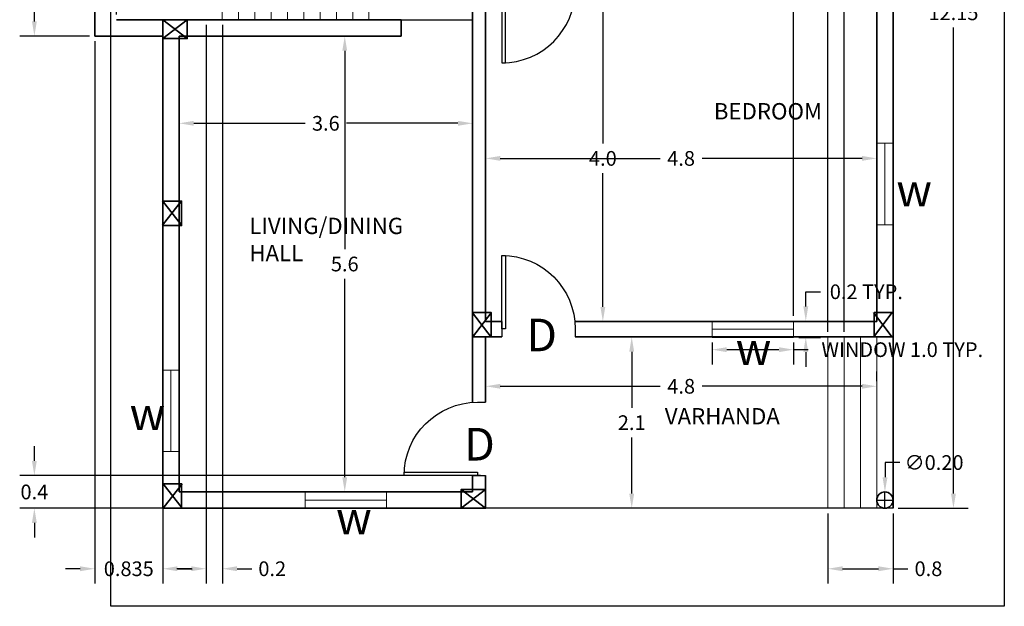
# Model space of a CAD drawing. Units: metres. Extents: x -16.7 to -4.6, y 24.4 to 40.
# Tile 1 of 2: x -16.7 to -4.6, y 24.4 to 31.6. Entities that reach past the tile are written whole.
import ezdxf

# ---------------------------------------------------------------- set-up
doc = ezdxf.new("R2010")
doc.units = ezdxf.units.M
doc.header["$MEASUREMENT"] = 0
doc.linetypes.add('ACAD_ISO02W100', pattern=[15, 12, -3])
for name, color, linetype, lineweight in [('A-ANNO-DIMS', 1, 'Continuous', 13), ('A-ANNO-TEXT', 5, 'Continuous', 18), ('A-ANNO-TTLB', 7, 'Continuous', 25), ('A-AREA-IDEN', 5, 'Continuous', 18), ('A-COLS', 7, 'Continuous', 35), ('A-FLOR', 4, 'Continuous', 25), ('A-WALL', 4, 'Continuous', 35), ('A-WALL-OVHD', 4, 'ACAD_ISO02W100', 25), ('door', 3, 'Continuous', 25), ('stair', 2, 'Continuous', 18), ('window', 6, 'Continuous', 20)]:
    doc.layers.add(name, color=color, linetype=linetype, lineweight=lineweight)
doc.styles.get("Standard").update_dxf_attribs({"font": 'arial.ttf'})
doc.dimstyles.get("Standard").update_dxf_attribs({"dimtxt": 0.18, "dimasz": 0.18, "dimexe": 0.18, "dimexo": 0.0625, "dimgap": 0.09, "dimtad": 0, "dimtih": 1, "dimtoh": 1, "dimdec": 1, "dimzin": 0, "dimdsep": 46, "dimtxsty": 'Standard', "dimcen": 0.09, "dimadec": 0, "dimazin": 0, "dimtfac": 1, "dimtdec": 1, "dimtofl": 0, "dimtmove": 0, "dimatfit": 3, "dimfxl": 1, "dimtolj": 1, "dimtzin": 0, "dimarcsym": 0})

# ---------------------------------------------------------------- blocks, each defined once
blk = doc.blocks.new('*U3')
for p, q in [((0, 0), (0, 100)), ((900, 0), (900, 100))]:
    blk.add_line(p, q)
blk.add_lwpolyline([(0, 0), (0, -900), (43.75, -900), (43.75, 0)], close=True)
blk.add_arc((0, 0), 900, 270, 0)
blk = doc.blocks.new('*U4')
for p, q in [((0, 0), (0, -100)), ((-900, 0), (-900, -100))]:
    blk.add_line(p, q)
blk.add_lwpolyline([(0, 0), (0, 900), (-43.75, 900), (-43.75, 0)], close=True)
blk.add_arc((0, 0), 900, 90, 180)
blk = doc.blocks.new('*D11')
at = {"layer": 'A-ANNO-DIMS', "color": 0, "lineweight": -2, "transparency": 16777216}
for p, q in [((-10.978, 29.979), (-10.978, 30.096)), ((-6.179, 29.979), (-6.179, 30.096)), ((-10.798, 29.916), (-8.836, 29.916)), ((-6.359, 29.916), (-8.321, 29.916))]:
    blk.add_line(p, q, dxfattribs=at)
at = {"layer": 'A-ANNO-DIMS', "color": 0, "transparency": 16777216}
for points in [[(-10.798, 29.946), (-10.798, 29.886), (-10.978, 29.916)], [(-6.359, 29.946), (-6.359, 29.886), (-6.179, 29.916)]]:
    blk.add_solid(points, dxfattribs=at)
at = {"layer": 'Defpoints', "color": 0, "transparency": 16777216}
for p in [(-10.978, 29.916), (-6.179, 29.916), (-6.179, 29.916)]:
    blk.add_point(p, dxfattribs=at)
at = {"layer": 'A-ANNO-DIMS', "color": 0, "transparency": 16777216, "insert": (-8.579, 29.916), "char_height": 0.18, "attachment_point": 5}
blk.add_mtext('\\A1;4.8', dxfattribs=at)
blk = doc.blocks.new('*D12')
at = {"layer": 'A-ANNO-DIMS', "color": 0, "lineweight": -2, "transparency": 16777216}
for p, q in [((-9.041, 31.916), (-9.719, 31.916)), ((-9.539, 31.736), (-9.539, 30.098)), ((-9.539, 28.096), (-9.539, 29.735)), ((-9.041, 27.916), (-9.719, 27.916))]:
    blk.add_line(p, q, dxfattribs=at)
at = {"layer": 'A-ANNO-DIMS', "color": 0, "transparency": 16777216}
for points in [[(-9.569, 31.736), (-9.509, 31.736), (-9.539, 31.916)], [(-9.569, 28.096), (-9.509, 28.096), (-9.539, 27.916)]]:
    blk.add_solid(points, dxfattribs=at)
at = {"layer": 'Defpoints', "color": 0, "transparency": 16777216}
for p in [(-8.978, 31.916), (-9.539, 27.916), (-8.978, 27.916)]:
    blk.add_point(p, dxfattribs=at)
at = {"layer": 'A-ANNO-DIMS', "color": 0, "transparency": 16777216, "insert": (-9.539, 29.916), "char_height": 0.18, "attachment_point": 5}
blk.add_mtext('\\A1;4.0', dxfattribs=at)
blk = doc.blocks.new('*D13')
at = {"layer": 'A-ANNO-DIMS', "color": 0, "lineweight": -2, "transparency": 16777216}
for p, q in [((-9.248, 27.726), (-9.365, 27.726)), ((-9.185, 27.546), (-9.185, 26.857)), ((-9.185, 25.806), (-9.185, 26.496)), ((-9.248, 25.626), (-9.365, 25.626))]:
    blk.add_line(p, q, dxfattribs=at)
at = {"layer": 'A-ANNO-DIMS', "color": 0, "transparency": 16777216}
for points in [[(-9.215, 27.546), (-9.155, 27.546), (-9.185, 27.726)], [(-9.215, 25.806), (-9.155, 25.806), (-9.185, 25.626)]]:
    blk.add_solid(points, dxfattribs=at)
at = {"layer": 'Defpoints', "color": 0, "transparency": 16777216}
for p in [(-9.185, 27.726), (-9.185, 25.626), (-9.185, 25.626)]:
    blk.add_point(p, dxfattribs=at)
at = {"layer": 'A-ANNO-DIMS', "color": 0, "transparency": 16777216, "insert": (-9.185, 26.676), "char_height": 0.18, "attachment_point": 5}
blk.add_mtext('\\A1;2.1', dxfattribs=at)
blk = doc.blocks.new('*D14')
at = {"layer": 'A-ANNO-DIMS', "color": 0, "lineweight": -2, "transparency": 16777216}
for p, q in [((-10.978, 27.185), (-10.978, 27.302)), ((-6.178, 27.185), (-6.178, 27.302)), ((-10.798, 27.122), (-8.836, 27.122)), ((-6.358, 27.122), (-8.321, 27.122))]:
    blk.add_line(p, q, dxfattribs=at)
at = {"layer": 'A-ANNO-DIMS', "color": 0, "transparency": 16777216}
for points in [[(-10.798, 27.152), (-10.798, 27.092), (-10.978, 27.122)], [(-6.358, 27.152), (-6.358, 27.092), (-6.178, 27.122)]]:
    blk.add_solid(points, dxfattribs=at)
at = {"layer": 'Defpoints', "color": 0, "transparency": 16777216}
for p in [(-10.978, 27.122), (-6.178, 27.122), (-6.178, 27.122)]:
    blk.add_point(p, dxfattribs=at)
at = {"layer": 'A-ANNO-DIMS', "color": 0, "transparency": 16777216, "insert": (-8.578, 27.122), "char_height": 0.18, "attachment_point": 5}
blk.add_mtext('\\A1;4.8', dxfattribs=at)
blk = doc.blocks.new('*D15')
at = {"layer": 'A-ANNO-DIMS', "color": 0, "lineweight": -2, "transparency": 16777216}
for p, q in [((-13.072, 31.416), (-12.526, 31.416)), ((-12.706, 31.236), (-12.706, 28.803)), ((-12.706, 26.006), (-12.706, 28.44)), ((-13.072, 25.826), (-12.526, 25.826))]:
    blk.add_line(p, q, dxfattribs=at)
at = {"layer": 'A-ANNO-DIMS', "color": 0, "transparency": 16777216}
for points in [[(-12.736, 31.236), (-12.676, 31.236), (-12.706, 31.416)], [(-12.736, 26.006), (-12.676, 26.006), (-12.706, 25.826)]]:
    blk.add_solid(points, dxfattribs=at)
at = {"layer": 'Defpoints', "color": 0, "transparency": 16777216}
for p in [(-13.135, 31.416), (-13.135, 25.826), (-12.706, 25.826)]:
    blk.add_point(p, dxfattribs=at)
at = {"layer": 'A-ANNO-DIMS', "color": 0, "transparency": 16777216, "insert": (-12.706, 28.621), "char_height": 0.18, "attachment_point": 5}
blk.add_mtext('\\A1;5.6', dxfattribs=at)
blk = doc.blocks.new('*D16')
at = {"layer": 'A-ANNO-DIMS', "color": 0, "lineweight": -2, "transparency": 16777216}
for p, q in [((-14.738, 30.098), (-14.738, 30.526)), ((-11.138, 30.098), (-11.138, 30.526)), ((-14.558, 30.346), (-13.192, 30.346)), ((-11.318, 30.346), (-12.685, 30.346))]:
    blk.add_line(p, q, dxfattribs=at)
at = {"layer": 'A-ANNO-DIMS', "color": 0, "transparency": 16777216}
for points in [[(-14.558, 30.376), (-14.558, 30.316), (-14.738, 30.346)], [(-11.318, 30.376), (-11.318, 30.316), (-11.138, 30.346)]]:
    blk.add_solid(points, dxfattribs=at)
at = {"layer": 'Defpoints', "color": 0, "transparency": 16777216}
for p in [(-11.138, 30.346), (-14.738, 30.036), (-11.138, 30.036)]:
    blk.add_point(p, dxfattribs=at)
at = {"layer": 'A-ANNO-DIMS', "color": 0, "transparency": 16777216, "insert": (-12.938, 30.346), "char_height": 0.18, "attachment_point": 5}
blk.add_mtext('\\A1;3.6', dxfattribs=at)
blk = doc.blocks.new('WIN-1000')
blk.add_line((0, 0.1), (1, 0.1))
blk.add_lwpolyline([(0, 0), (1, 0), (1, 0.2), (0, 0.2)], close=True)
blk = doc.blocks.new('COL-300x230')
for p, q in [((0, 0.23), (0.3, 0)), ((0, 0), (0.3, 0.23))]:
    blk.add_line(p, q)
blk.add_lwpolyline([(0, 0), (0, 0.23), (0.3, 0.23), (0.3, 0)], close=True)
blk = doc.blocks.new('STAIR-FLIGHT-2000x900')
for p, q in [((0.2, 0.9), (0.2, 0)), ((0.4, 0.9), (0.4, 0)), ((0.6, 0.9), (0.6, 0)), ((0.8, 0.9), (0.8, 0)), ((1, 0.9), (1, 0)), ((1.2, 0.9), (1.2, 0)), ((1.4, 0.9), (1.4, 0)), ((1.6, 0.9), (1.6, 0)), ((1.8, 0.9), (1.8, 0)), ((2, 0.9), (2, 0)), ((2, 0), (0, 0))]:
    blk.add_line(p, q)
blk = doc.blocks.new('*D23')
at = {"layer": 'A-ANNO-DIMS', "color": 0, "lineweight": -2, "transparency": 16777216}
for p, q in [((-8.199, 27.659), (-8.199, 27.391)), ((-8.019, 27.571), (-7.379, 27.571)), ((-7.199, 27.659), (-7.199, 27.391)), ((-7.199, 27.571), (-7.019, 27.571))]:
    blk.add_line(p, q, dxfattribs=at)
at = {"layer": 'A-ANNO-DIMS', "color": 0, "transparency": 16777216}
for points in [[(-8.019, 27.601), (-8.019, 27.541), (-8.199, 27.571)], [(-7.379, 27.601), (-7.379, 27.541), (-7.199, 27.571)]]:
    blk.add_solid(points, dxfattribs=at)
at = {"layer": 'Defpoints', "color": 0, "transparency": 16777216}
for p in [(-8.199, 27.721), (-7.199, 27.721), (-7.199, 27.571)]:
    blk.add_point(p, dxfattribs=at)
at = {"layer": 'A-ANNO-DIMS', "color": 0, "transparency": 16777216, "insert": (-5.865, 27.571), "char_height": 0.18, "attachment_point": 5}
blk.add_mtext('\\A1;WINDOW 1.0 TYP.', dxfattribs=at)
blk = doc.blocks.new('*D24')
at = {"layer": 'A-ANNO-DIMS', "color": 0, "lineweight": -2, "transparency": 16777216}
for p, q in [((-7.049, 28.101), (-7.049, 28.281)), ((-7.049, 28.281), (-6.869, 28.281)), ((-7.136, 27.921), (-6.869, 27.921)), ((-7.136, 27.721), (-6.869, 27.721)), ((-7.049, 27.541), (-7.049, 27.361))]:
    blk.add_line(p, q, dxfattribs=at)
at = {"layer": 'A-ANNO-DIMS', "color": 0, "transparency": 16777216}
for points in [[(-7.079, 28.101), (-7.019, 28.101), (-7.049, 27.921)], [(-7.079, 27.541), (-7.019, 27.541), (-7.049, 27.721)]]:
    blk.add_solid(points, dxfattribs=at)
at = {"layer": 'Defpoints', "color": 0, "transparency": 16777216}
for p in [(-7.199, 27.921), (-7.049, 27.921), (-7.199, 27.721)]:
    blk.add_point(p, dxfattribs=at)
at = {"layer": 'A-ANNO-DIMS', "color": 0, "transparency": 16777216, "insert": (-6.306, 28.281), "char_height": 0.18, "attachment_point": 5}
blk.add_mtext('\\A1;0.2 TYP.', dxfattribs=at)
blk = doc.blocks.new('*D32')
at = {"layer": 'A-ANNO-DIMS', "color": 0, "lineweight": -2, "transparency": 16777216}
for p, q in [((-5.916, 37.776), (-5.057, 37.776)), ((-5.237, 37.596), (-5.237, 31.883)), ((-5.237, 25.806), (-5.237, 31.52)), ((-5.916, 25.626), (-5.057, 25.626))]:
    blk.add_line(p, q, dxfattribs=at)
at = {"layer": 'A-ANNO-DIMS', "color": 0, "transparency": 16777216}
for points in [[(-5.267, 37.596), (-5.207, 37.596), (-5.237, 37.776)], [(-5.267, 25.806), (-5.207, 25.806), (-5.237, 25.626)]]:
    blk.add_solid(points, dxfattribs=at)
at = {"layer": 'Defpoints', "color": 0, "transparency": 16777216}
for p in [(-5.978, 37.776), (-5.237, 37.776), (-5.978, 25.626)]:
    blk.add_point(p, dxfattribs=at)
at = {"layer": 'A-ANNO-DIMS', "color": 0, "transparency": 16777216, "insert": (-5.237, 31.701), "char_height": 0.18, "attachment_point": 5}
blk.add_mtext('\\A1;12.15', dxfattribs=at)
blk = doc.blocks.new('*D33')
at = {"layer": 'A-ANNO-DIMS', "color": 0, "lineweight": -2, "transparency": 16777216}
for p, q in [((-15.773499, 31.353944), (-15.773499, 24.704754)), ((-14.938499, 31.353944), (-14.938499, 24.704754)), ((-15.953499, 24.884754), (-16.133499, 24.884754)), ((-14.758499, 24.884754), (-14.578499, 24.884754))]:
    blk.add_line(p, q, dxfattribs=at)
at = {"layer": 'A-ANNO-DIMS', "color": 0, "transparency": 16777216}
for points in [[(-15.953499, 24.914754), (-15.953499, 24.854754), (-15.773499, 24.884754)], [(-14.758499, 24.914754), (-14.758499, 24.854754), (-14.938499, 24.884754)]]:
    blk.add_solid(points, dxfattribs=at)
at = {"layer": 'Defpoints', "color": 0, "transparency": 16777216}
for p in [(-15.773499, 31.416444), (-14.938499, 31.416444), (-15.773499, 24.884754)]:
    blk.add_point(p, dxfattribs=at)
at = {"layer": 'A-ANNO-DIMS', "color": 0, "transparency": 16777216, "insert": (-15.355999, 24.884754), "char_height": 0.18, "attachment_point": 5}
blk.add_mtext('\\A1;0.835', dxfattribs=at)
blk = doc.blocks.new('*D34')
at = {"layer": 'A-ANNO-DIMS', "color": 0, "lineweight": -2, "transparency": 16777216}
for p, q in [((-15.836, 33.816), (-16.694, 33.816)), ((-16.514, 33.636), (-16.514, 32.797)), ((-16.514, 31.596), (-16.514, 32.436)), ((-15.836, 31.416), (-16.694, 31.416))]:
    blk.add_line(p, q, dxfattribs=at)
at = {"layer": 'A-ANNO-DIMS', "color": 0, "transparency": 16777216}
for points in [[(-16.544, 33.636), (-16.484, 33.636), (-16.514, 33.816)], [(-16.544, 31.596), (-16.484, 31.596), (-16.514, 31.416)]]:
    blk.add_solid(points, dxfattribs=at)
at = {"layer": 'Defpoints', "color": 0, "transparency": 16777216}
for p in [(-16.514, 33.816), (-15.773, 33.816), (-15.773, 31.416)]:
    blk.add_point(p, dxfattribs=at)
at = {"layer": 'A-ANNO-DIMS', "color": 0, "transparency": 16777216, "insert": (-16.514, 32.616), "char_height": 0.18, "attachment_point": 5}
blk.add_mtext('\\A1;2.4', dxfattribs=at)
blk = doc.blocks.new('*D35')
at = {"layer": 'A-ANNO-DIMS', "color": 0, "lineweight": -2, "transparency": 16777216}
for p, q in [((-15.508, 31.679), (-15.508, 38.697)), ((-14.408, 32.749), (-14.408, 38.697)), ((-15.328, 38.517), (-15.187, 38.517)), ((-14.588, 38.517), (-14.73, 38.517))]:
    blk.add_line(p, q, dxfattribs=at)
at = {"layer": 'A-ANNO-DIMS', "color": 0, "transparency": 16777216}
for points in [[(-15.328, 38.547), (-15.328, 38.487), (-15.508, 38.517)], [(-14.588, 38.547), (-14.588, 38.487), (-14.408, 38.517)]]:
    blk.add_solid(points, dxfattribs=at)
at = {"layer": 'Defpoints', "color": 0, "transparency": 16777216}
for p in [(-14.408, 38.517), (-14.408, 32.686), (-15.508, 31.616)]:
    blk.add_point(p, dxfattribs=at)
at = {"layer": 'A-ANNO-DIMS', "color": 0, "transparency": 16777216, "insert": (-14.958, 38.517), "char_height": 0.18, "attachment_point": 5}
blk.add_mtext('\\A1;1.1', dxfattribs=at)
blk = doc.blocks.new('*D36')
at = {"layer": 'A-ANNO-DIMS', "color": 0, "lineweight": -2, "transparency": 16777216}
for p, q in [((-14.408, 31.554), (-14.408, 24.705)), ((-14.208, 31.554), (-14.208, 24.705)), ((-14.588, 24.885), (-14.768, 24.885)), ((-14.028, 24.885), (-13.848, 24.885))]:
    blk.add_line(p, q, dxfattribs=at)
at = {"layer": 'A-ANNO-DIMS', "color": 0, "transparency": 16777216}
for points in [[(-14.588, 24.915), (-14.588, 24.855), (-14.408, 24.885)], [(-14.028, 24.915), (-14.028, 24.855), (-14.208, 24.885)]]:
    blk.add_solid(points, dxfattribs=at)
at = {"layer": 'Defpoints', "color": 0, "transparency": 16777216}
for p in [(-14.408, 31.616), (-14.208, 31.616), (-14.208, 24.885)]:
    blk.add_point(p, dxfattribs=at)
at = {"layer": 'A-ANNO-DIMS', "color": 0, "transparency": 16777216, "insert": (-13.596, 24.885), "char_height": 0.18, "attachment_point": 5}
blk.add_mtext('\\A1;0.2', dxfattribs=at)
blk = doc.blocks.new('*D37')
at = {"layer": 'A-ANNO-DIMS', "color": 0, "lineweight": -2, "transparency": 16777216}
for p, q in [((-6.778, 25.564), (-6.778, 24.705)), ((-5.978, 25.564), (-5.978, 24.705)), ((-6.598, 24.885), (-6.158, 24.885)), ((-5.978, 24.885), (-5.798, 24.885))]:
    blk.add_line(p, q, dxfattribs=at)
at = {"layer": 'A-ANNO-DIMS', "color": 0, "transparency": 16777216}
for points in [[(-6.598, 24.915), (-6.598, 24.855), (-6.778, 24.885)], [(-6.158, 24.915), (-6.158, 24.855), (-5.978, 24.885)]]:
    blk.add_solid(points, dxfattribs=at)
at = {"layer": 'Defpoints', "color": 0, "transparency": 16777216}
for p in [(-6.778, 25.626), (-5.978, 25.626), (-5.978, 24.885)]:
    blk.add_point(p, dxfattribs=at)
at = {"layer": 'A-ANNO-DIMS', "color": 0, "transparency": 16777216, "insert": (-5.544, 24.885), "char_height": 0.18, "attachment_point": 5}
blk.add_mtext('\\A1;0.8', dxfattribs=at)
blk = doc.blocks.new('*D38')
at = {"layer": 'A-ANNO-DIMS', "color": 0, "lineweight": -2, "transparency": 16777216}
for p, q in [((-6.778, 27.789), (-6.778, 38.697)), ((-6.578, 27.789), (-6.578, 38.697)), ((-6.958, 38.517), (-7.138, 38.517)), ((-6.398, 38.517), (-6.218, 38.517))]:
    blk.add_line(p, q, dxfattribs=at)
at = {"layer": 'A-ANNO-DIMS', "color": 0, "transparency": 16777216}
for points in [[(-6.958, 38.547), (-6.958, 38.487), (-6.778, 38.517)], [(-6.398, 38.547), (-6.398, 38.487), (-6.578, 38.517)]]:
    blk.add_solid(points, dxfattribs=at)
at = {"layer": 'Defpoints', "color": 0, "transparency": 16777216}
for p in [(-6.578, 38.517), (-6.778, 27.726), (-6.578, 27.726)]:
    blk.add_point(p, dxfattribs=at)
at = {"layer": 'A-ANNO-DIMS', "color": 0, "transparency": 16777216, "insert": (-5.966, 38.517), "char_height": 0.18, "attachment_point": 5}
blk.add_mtext('\\A1;0.2', dxfattribs=at)
blk = doc.blocks.new('*D39')
at = {"layer": 'A-ANNO-DIMS', "color": 0, "lineweight": -2, "transparency": 16777216}
for p, q in [((-7.199, 27.984), (-7.199, 38.697)), ((-6.178, 27.979), (-6.178, 38.697)), ((-7.379, 38.517), (-7.559, 38.517)), ((-5.998, 38.517), (-5.818, 38.517))]:
    blk.add_line(p, q, dxfattribs=at)
at = {"layer": 'A-ANNO-DIMS', "color": 0, "transparency": 16777216}
for points in [[(-7.379, 38.547), (-7.379, 38.487), (-7.199, 38.517)], [(-5.998, 38.547), (-5.998, 38.487), (-6.178, 38.517)]]:
    blk.add_solid(points, dxfattribs=at)
at = {"layer": 'Defpoints', "color": 0, "transparency": 16777216}
for p in [(-7.199, 38.517), (-7.199, 27.921), (-6.178, 27.916)]:
    blk.add_point(p, dxfattribs=at)
at = {"layer": 'A-ANNO-DIMS', "color": 0, "transparency": 16777216, "insert": (-6.689, 38.517), "char_height": 0.18, "attachment_point": 5}
blk.add_mtext('\\A1;1.02', dxfattribs=at)
blk = doc.blocks.new('*D40')
at = {"layer": 'A-ANNO-DIMS', "color": 0, "lineweight": -2, "transparency": 16777216}
for p, q in [((-16.514499, 26.206444), (-16.514499, 26.386444)), ((-11.040999, 26.026444), (-16.694499, 26.026444)), ((-11.040999, 25.626444), (-16.694499, 25.626444)), ((-16.514499, 25.446444), (-16.514499, 25.266444))]:
    blk.add_line(p, q, dxfattribs=at)
at = {"layer": 'A-ANNO-DIMS', "color": 0, "transparency": 16777216}
for points in [[(-16.544499, 26.206444), (-16.484499, 26.206444), (-16.514499, 26.026444)], [(-16.544499, 25.446444), (-16.484499, 25.446444), (-16.514499, 25.626444)]]:
    blk.add_solid(points, dxfattribs=at)
at = {"layer": 'Defpoints', "color": 0, "transparency": 16777216}
for p in [(-16.514499, 26.026444), (-10.978499, 26.026444), (-10.978499, 25.626444)]:
    blk.add_point(p, dxfattribs=at)
at = {"layer": 'A-ANNO-DIMS', "color": 0, "transparency": 16777216, "insert": (-16.514499, 25.826444), "char_height": 0.18, "attachment_point": 5}
blk.add_mtext('\\A1;0.4', dxfattribs=at)
blk = doc.blocks.new('*D44')
at = {"layer": 'A-ANNO-DIMS', "color": 0, "lineweight": -2, "transparency": 16777216}
for p, q in [((-6.076, 26.187), (-6.077, 26.007)), ((-5.896, 26.187), (-6.076, 26.187)), ((-6.078, 25.637), (-6.078, 25.817)), ((-6.168, 25.727), (-5.988, 25.727))]:
    blk.add_line(p, q, dxfattribs=at)
at = {"layer": 'A-ANNO-DIMS', "color": 0, "transparency": 16777216}
blk.add_solid([(-6.107, 26.007), (-6.047, 26.006), (-6.078, 25.827)], dxfattribs=at)
at = {"layer": 'Defpoints', "color": 0, "transparency": 16777216}
for p in [(-6.078, 25.827), (-6.079, 25.626)]:
    blk.add_point(p, dxfattribs=at)
at = {"layer": 'A-ANNO-DIMS', "color": 0, "transparency": 16777216, "insert": (-5.475, 26.187), "char_height": 0.18, "attachment_point": 5}
blk.add_mtext('\\A1;∅0.20', dxfattribs=at)

msp = doc.modelspace()

# ---------------------------------------------------------------- linework, layer by layer
at = {"layer": 'A-ANNO-TTLB'}
msp.add_lwpolyline([(-15.5749, 40.0289), (-4.6131, 40.0289), (-4.6131, 24.4246), (-15.5749, 24.4246)], close=True, dxfattribs=at)
at = {"layer": 'A-COLS'}
for p, q in [((-14.9393, 31.6146), (-14.6393, 31.3846)), ((-14.9393, 31.3846), (-14.6393, 31.6146)), ((-14.9403, 29.0962), (-14.7103, 29.3962)), ((-14.9403, 29.3962), (-14.7103, 29.0962)), ((-11.138, 27.7241), (-10.908, 28.0241)), ((-11.138, 28.0241), (-10.908, 27.7241)), ((-6.2183, 27.7262), (-5.9883, 28.0262)), ((-6.2183, 28.0262), (-5.9883, 27.7262)), ((-14.9328, 25.6258), (-14.7028, 25.9258)), ((-14.9328, 25.9258), (-14.7028, 25.6258))]:
    msp.add_line(p, q, dxfattribs=at)
for points in [[(-14.9386, 31.385), (-14.9386, 31.615), (-14.6386, 31.615), (-14.6386, 31.385)], [(-14.9385, 29.3932), (-14.7085, 29.3932), (-14.7085, 29.0932), (-14.9385, 29.0932)], [(-10.9085, 27.7264), (-11.1385, 27.7264), (-11.1385, 28.0264), (-10.9085, 28.0264)], [(-6.2085, 28.0264), (-5.9785, 28.0264), (-5.9785, 27.7264), (-6.2085, 27.7264)], [(-14.7085, 25.6264), (-14.9385, 25.6264), (-14.9385, 25.9264), (-14.7085, 25.9264)]]:
    msp.add_lwpolyline(points, close=True, dxfattribs=at)
msp.add_circle((-6.0785, 25.7265), 0.1001, dxfattribs=at)
at = {"layer": 'A-FLOR'}
msp.add_line((-5.9785, 25.6264), (-10.9785, 25.6264), dxfattribs=at)
at = {"layer": 'A-WALL'}
for p, q in [((-15.7735, 31.4164), (-15.7735, 33.8164)), ((-11.1385, 31.6164), (-11.1385, 32.0864)), ((-5.9785, 32.0864), (-5.9785, 25.6264)), ((-15.5085, 31.6164), (-14.7385, 31.6164)), ((-14.9385, 31.6164), (-12.0119, 31.6164)), ((-12.0119, 31.4164), (-12.0119, 31.6164)), ((-11.1385, 26.9244), (-11.1385, 31.6164)), ((-15.7735, 31.4164), (-14.9385, 31.4164)), ((-14.9385, 25.6264), (-14.9385, 31.4164)), ((-14.7385, 25.8264), (-14.7385, 31.4164)), ((-14.7385, 31.4164), (-12.0119, 31.4164)), ((-11.1385, 31.2164), (-11.1385, 26.9244)), ((-10.9785, 27.7264), (-10.7785, 27.7264)), ((-10.7785, 27.7264), (-10.9785, 27.7264)), ((-10.9785, 26.9264), (-10.9785, 27.7264)), ((-6.1785, 27.7264), (-9.8785, 27.7264)), ((-9.8785, 27.7264), (-6.1785, 27.7264)), ((-11.1385, 25.8264), (-11.1385, 26.0264)), ((-11.1385, 26.0264), (-11.1385, 25.8264)), ((-10.9785, 25.6264), (-10.9785, 26.0264)), ((-11.1385, 25.8264), (-14.7385, 25.8264)), ((-10.9785, 25.6264), (-14.9385, 25.6264)), ((-11.1385, 25.6264), (-14.9385, 25.6264))]:
    msp.add_line(p, q, dxfattribs=at)
for points in [[(-10.7785, 27.9164), (-10.9785, 27.9164), (-10.9785, 31.9164), (-10.7785, 31.9164)], [(-9.8812, 31.9164), (-6.1785, 31.9164), (-6.1785, 27.9164), (-9.883, 27.9164)]]:
    msp.add_lwpolyline(points, dxfattribs=at)
at = {"layer": 'A-WALL-OVHD', "ltscale": 1.2}
msp.add_line((-12.0119, 31.6164), (-11.1385, 31.6164), dxfattribs=at)
at = {"layer": 'door'}
for p, q in [((-10.7785, 27.9164), (-10.7785, 27.7264)), ((-11.1385, 26.0264), (-10.9785, 26.0264))]:
    msp.add_line(p, q, dxfattribs=at)
at = {"layer": 'stair'}
for p, q in [((-6.7785, 27.7264), (-6.7785, 25.6264)), ((-6.5785, 27.7264), (-6.5785, 25.6264)), ((-6.3785, 27.7264), (-6.3785, 25.6264)), ((-6.1785, 27.7264), (-6.1785, 25.6264))]:
    msp.add_line(p, q, dxfattribs=at)

# ---------------------------------------------------------------- block references
at = {"layer": 'A-COLS'}
msp.add_blockref('COL-300x230', (-11.2785, 25.6264), dxfattribs=at)
at = {"layer": 'door', "yscale": 0.001, "zscale": 0.001}
for name, p, xscale in [('*U3', (-10.7785, 31.9864), 0.001), ('*U4', (-10.7785, 27.8264), -0.001)]:
    msp.add_blockref(name, p, dxfattribs=dict(at, xscale=xscale))
at = {"layer": 'door', "xscale": -0.001, "yscale": 0.001, "zscale": 0.001, "rotation": 90}
msp.add_blockref('*U4', (-11.0785, 26.0264), dxfattribs=at)
at = {"layer": 'stair', "extrusion": (0, 0, -1), "zscale": -1, "rotation": 180}
msp.add_blockref('STAIR-FLIGHT-2000x900', (14.4085, 32.5164), dxfattribs=at)
at = {"layer": 'window', "rotation": 89.99999999999946}
for p in [(-5.9786, 29.1034), (-14.7385, 26.3214)]:
    msp.add_blockref('WIN-1000', p, dxfattribs=at)
at = {"layer": 'window'}
for p in [(-8.1985, 27.7212), (-13.1919, 25.6264)]:
    msp.add_blockref('WIN-1000', p, dxfattribs=at)

# ---------------------------------------------------------------- texts
at = {"layer": 'A-ANNO-TEXT', "char_height": 0.4, "attachment_point": 1}
for s, insert in [('w', (-5.9382, 29.7272)), ('D', (-10.4774, 27.951)), ('w', (-7.9094, 27.7821)), ('w', (-15.3461, 26.9841)), ('D', (-11.2398, 26.6114)), ('w', (-12.8129, 25.7075))]:
    msp.add_mtext_dynamic_manual_height_columns(s, width=0.312835, gutter_width=1, heights=[0], dxfattribs=dict(at, insert=insert))
at = {"layer": 'A-AREA-IDEN', "char_height": 0.2, "attachment_point": 1}
for s, insert in [('BEDROOM', (-8.1766, 30.5941)), ('LIVING/DINING HALL', (-13.8771, 29.1883)), ('VARHANDA', (-8.7791, 26.8548))]:
    msp.add_mtext_dynamic_manual_height_columns(s, width=0.273342, gutter_width=1, heights=[0], dxfattribs=dict(at, insert=insert))

# ---------------------------------------------------------------- dimensions: what is measured, and where the dimension line sits
at = {"layer": 'A-ANNO-DIMS'}
for base, p1, p2, override, picture, middle in [((-14.4085, 38.5174), (-15.5085, 31.6164), (-14.4085, 32.6864), {"dimdec": 1, "dimlfac": 1, "dimrnd": 0, "dimzin": 0, "dimdsep": 46, "dimlunit": 2}, '*D35', (-14.9585, 38.5174)), ((-7.1986, 38.5174), (-6.1785, 27.9164), (-7.1986, 27.9212), {"dimdec": 2, "dimlfac": 1, "dimrnd": 0, "dimzin": 0, "dimdsep": 46, "dimlunit": 2}, '*D39', (-6.6885, 38.5174)), ((-6.5785, 38.5174), (-6.7785, 27.7264), (-6.5785, 27.7264), {"dimdec": 1, "dimlfac": 1, "dimrnd": 0, "dimzin": 0, "dimdsep": 46, "dimlunit": 2}, '*D38', (-5.9656, 38.5174)), ((-14.2085, 24.8848), (-14.4085, 31.6164), (-14.2085, 31.6164), {"dimdec": 1, "dimlfac": 1, "dimrnd": 0, "dimzin": 0, "dimdsep": 46, "dimlunit": 2}, '*D36', (-13.5956, 24.8848)), ((-15.7735, 24.8848), (-14.9385, 31.4164), (-15.7735, 31.4164), {"dimdec": 3, "dimlfac": 1, "dimrnd": 0, "dimzin": 0, "dimdsep": 46, "dimlunit": 2}, '*D33', (-15.356, 24.8848)), ((-11.1385, 30.3456), (-14.7385, 30.0355), (-11.1385, 30.0355), {"dimclrd": 0, "dimclre": 0, "dimclrt": 0}, '*D16', (-12.9385, 30.3456)), ((-6.1786, 29.9164), (-10.9785, 29.9164), (-6.1786, 29.9164), {"dimclrd": 0, "dimclre": 0, "dimclrt": 0}, '*D11', (-8.5785, 29.9164)), ((-6.1785, 27.1224), (-10.9785, 27.1224), (-6.1785, 27.1224), {"dimclrd": 0, "dimclre": 0, "dimclrt": 0}, '*D14', (-8.5785, 27.1224)), ((-5.9785, 24.8848), (-6.7785, 25.6264), (-5.9785, 25.6264), {"dimdec": 1, "dimlfac": 1, "dimrnd": 0, "dimzin": 0, "dimdsep": 46, "dimlunit": 2}, '*D37', (-5.5445, 24.8848))]:
    dim = msp.add_linear_dim(base=base, p1=p1, p2=p2, dimstyle='Standard', override=override, dxfattribs=at)
    dim.commit()
    dim.dimension.update_dxf_attribs({"geometry": picture, "text_midpoint": middle})
for base, p1, p2, override, picture, middle in [((-5.237, 37.7764), (-5.9785, 25.6264), (-5.9783, 37.7764), {"dimdec": 2, "dimlfac": 1, "dimrnd": 0, "dimzin": 0, "dimdsep": 46, "dimlunit": 2}, '*D32', (-5.237, 31.7014)), ((-16.5145, 33.8164), (-15.7735, 31.4164), (-15.7735, 33.8164), {"dimdec": 1, "dimlfac": 1, "dimrnd": 0, "dimzin": 0, "dimdsep": 46, "dimlunit": 2}, '*D34', (-16.5145, 32.6164)), ((-9.5386, 27.9164), (-8.9785, 31.9164), (-8.9785, 27.9164), {"dimclrd": 0, "dimclre": 0, "dimclrt": 0}, '*D12', (-9.5386, 29.9164)), ((-12.7056, 25.8264), (-13.1347, 31.4164), (-13.1347, 25.8264), {"dimclrd": 0, "dimclre": 0, "dimclrt": 0}, '*D15', (-12.7056, 28.6214)), ((-9.1853, 25.6264), (-9.1853, 27.7264), (-9.1853, 25.6264), {"dimclrd": 0, "dimclre": 0, "dimclrt": 0}, '*D13', (-9.1853, 26.6764)), ((-16.5145, 26.0264), (-10.9785, 25.6264), (-10.9785, 26.0264), {"dimdec": 1, "dimlfac": 1, "dimrnd": 0, "dimzin": 0, "dimdsep": 46, "dimlunit": 2}, '*D40', (-16.5145, 25.8264))]:
    dim = msp.add_linear_dim(base=base, p1=p1, p2=p2, angle=90, dimstyle='Standard', override=override, dxfattribs=at)
    dim.commit()
    dim.dimension.update_dxf_attribs({"geometry": picture, "text_midpoint": middle})
dim = msp.add_linear_dim(base=(-7.0485, 27.9212), p1=(-7.1986, 27.7212), p2=(-7.1986, 27.9212), angle=90, text='<> TYP.', dimstyle='Standard', override={"dimdec": 1, "dimlfac": 1, "dimrnd": 0, "dimzin": 0, "dimdsep": 46, "dimlunit": 2}, dxfattribs=at)
dim.commit()
dim.dimension.update_dxf_attribs({"geometry": '*D24', "text_midpoint": (-6.3055, 28.2812)})
dim = msp.add_linear_dim(base=(-7.1986, 27.5712), p1=(-8.1985, 27.7212), p2=(-7.1986, 27.7212), text='WINDOW <> TYP.', dimstyle='Standard', override={"dimdec": 1, "dimlfac": 1, "dimrnd": 0, "dimzin": 0, "dimdsep": 46, "dimlunit": 2}, dxfattribs=at)
dim.commit()
dim.dimension.update_dxf_attribs({"geometry": '*D23', "text_midpoint": (-5.8652, 27.5712)})
dim = msp.add_diameter_dim_2p(p1=(-6.079, 25.6264), p2=(-6.078, 25.8266), dimstyle='Standard', override={"dimdec": 2, "dimlfac": 1, "dimrnd": 0, "dimzin": 0, "dimdsep": 46, "dimlunit": 2}, dxfattribs=at)
dim.commit()
dim.dimension.update_dxf_attribs({"geometry": '*D44', "text_midpoint": (-5.4748, 26.1866), "dimtype": 163})

doc.saveas('drawing.dxf')
